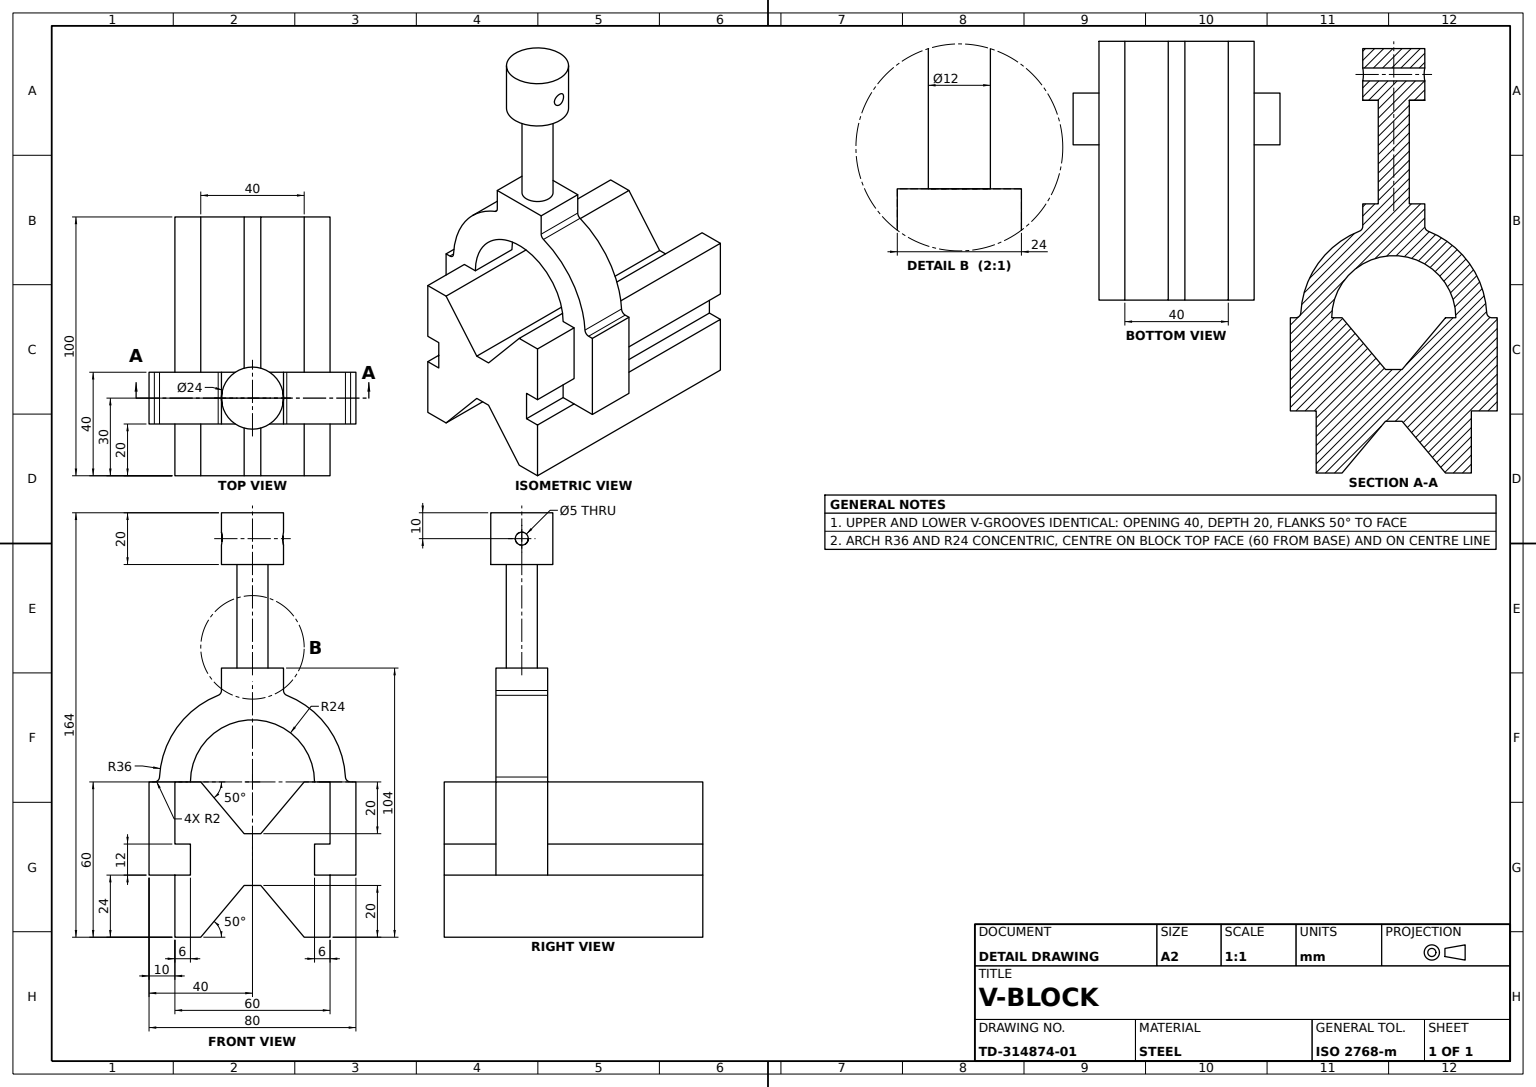
from build123d import *

# Parameters (mm, degrees)
V_BLOCK_BASE_DEPTH         = 70
V_BLOCK_BASE_DEPTH_BACK    = 30
CLAMP_ARCH_DEPTH           = 10
CLAMP_ARCH_FILLET_R2_R     = 2
CLAMP_SCREW_SKETCH_R       = 6
CLAMP_SCREW_SHAFT_DEPTH    = 60
CLAMP_START                = 40
SKETCH4_3_R                = 12
SKETCH4_3_R_2              = 6
CLAMP_SCREW_KNOB_DEPTH     = 20
KNOB_CROSS_HOLE_DEPTH      = 157.384142419
KNOB_CROSS_HOLE_DEPTH_BACK = 157.384142419
KNOB_CROSS_HOLE_SKETCH_R   = 2.5


with BuildPart() as part:
    # V-Block Profile Sketch → V-Block Base (new, two sides: drawn at the far end of the back side and taken through both)
    with BuildSketch(Plane.XY.offset(-V_BLOCK_BASE_DEPTH_BACK)):
        Polygon((-24, -6), (-30, -6), (-30, -30), (-20, -30), (-3.218007376, -10), (3.218007376, -10), (20, -30), (30, -30), (30, -6), (24, -6), (24, 6), (30, 6), (30, 30), (20, 30), (3.218007376, 10), (-3.218007376, 10), (-20, 30), (-30, 30), (-30, 6), (-24, 6), align=None)
    extrude(amount=V_BLOCK_BASE_DEPTH + V_BLOCK_BASE_DEPTH_BACK)

    # Clamp Arch Sketch → Clamp Arch (add, symmetric)
    with BuildSketch(Plane.XY):
        with BuildLine():
            Line((-40, -6), (40, -6))
            Line((40, -6), (40, 30))
            Line((40, 30), (36, 30))
            ThreePointArc((36, 30), (29.393876913, 50.784609691), (12, 63.941125497))
            Line((12, 63.941125497), (12, 74))
            Line((12, 74), (-12, 74))
            Line((-12, 74), (-12, 63.941125497))
            ThreePointArc((-12, 63.941125497), (-29.393876913, 50.784609691), (-36, 30))
            Line((-36, 30), (-40, 30))
            Line((-40, 30), (-40, -6))
        make_face()
        with BuildLine():
            Line((-20, 30), (-24, 30))
            ThreePointArc((-24, 30), (0, 54), (24, 30))
            Line((24, 30), (20, 30))
            Line((20, 30), (3.218007376, 10))
            Line((3.218007376, 10), (-3.218007376, 10))
            Line((-3.218007376, 10), (-20, 30))
        make_face(mode=Mode.SUBTRACT)
    extrude(amount=CLAMP_ARCH_DEPTH, both=True)

    # Clamp Arch Fillet R2
    clamp_arch_fillet_r2_edges = [part.edges().sort_by_distance(p)[0] for p in [
        (36, 30, 0),
        (12, 63.941125497, 0),
        (-12, 63.941125497, 0),
        (-36, 30, 0),
    ]]
    fillet(clamp_arch_fillet_r2_edges, radius=CLAMP_ARCH_FILLET_R2_R)

    # Clamp Screw Sketch → Clamp Screw Shaft (add)
    with BuildSketch(Plane(origin=(0, 74, 0), x_dir=(1, 0, 0), z_dir=(0, 1, 0))):
        with Locations(Location((0, 0, 0), (0, 0, 270))):
            Circle(CLAMP_SCREW_SKETCH_R)
    extrude(amount=CLAMP_SCREW_SHAFT_DEPTH)

    # Sketch4_3 → Clamp Screw Knob (add)
    with BuildSketch(Plane(origin=(0, 74, 0), x_dir=(1, 0, 0), z_dir=(0, 1, 0)).offset(CLAMP_START)):
        with Locations(Location((0, 0, 0), (0, 0, 270))):
            Circle(SKETCH4_3_R)
        with Locations(Location((0, 0, 0), (0, 0, 270))):
            Circle(SKETCH4_3_R_2, mode=Mode.SUBTRACT)
    extrude(amount=CLAMP_SCREW_KNOB_DEPTH)

    # Knob Cross Hole Sketch → Knob Cross Hole (cut, two sides: drawn at the far end of the back side and taken through both)
    with BuildSketch(Plane(origin=(0, 0, 0), x_dir=(0, 0, -1), z_dir=(1, 0, 0)).offset(-KNOB_CROSS_HOLE_DEPTH_BACK)):
        with Locations((0, 124)):
            Circle(KNOB_CROSS_HOLE_SKETCH_R)
    extrude(amount=KNOB_CROSS_HOLE_DEPTH + KNOB_CROSS_HOLE_DEPTH_BACK, mode=Mode.SUBTRACT)


solid = part.part
